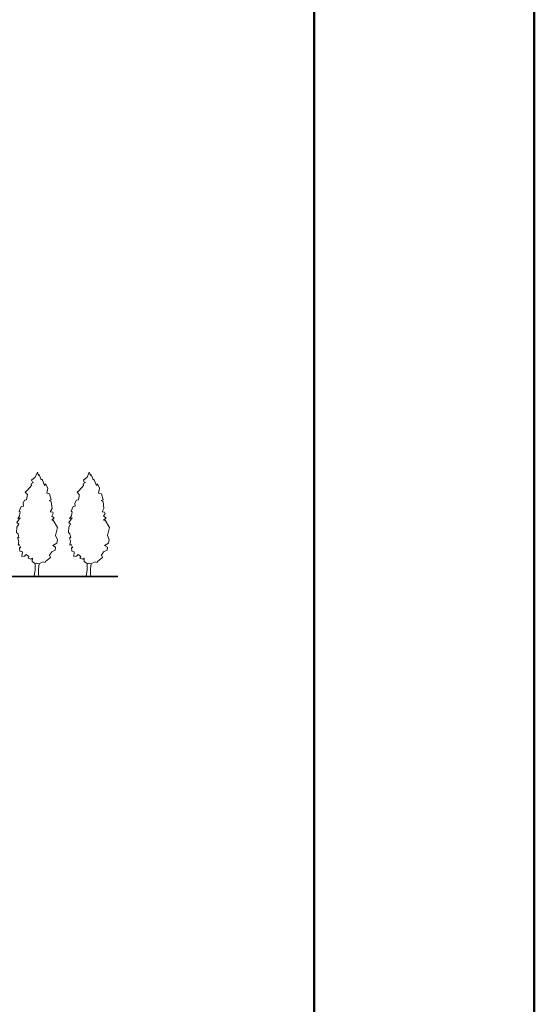
# Model space of a CAD drawing. Units: inches. Extents: x -1080 to 1950, y -1929 to 857.
# Tile 12 of 16: x 1630 to 1950, y -1001 to -389. Entities that reach past the tile are written whole.
import ezdxf

# ---------------------------------------------------------------- set-up
doc = ezdxf.new("R2010")
doc.units = ezdxf.units.IN
doc.header["$MEASUREMENT"] = 0
for name, color, linetype, lineweight in [('A-ANNO-TTLB', 7, 'Continuous', 50), ('A-ELEV', 7, 'Continuous', 35), ('L-PLNT', 82, 'Continuous', 13)]:
    doc.layers.add(name, color=color, linetype=linetype, lineweight=lineweight)

# ---------------------------------------------------------------- blocks, each defined once
blk = doc.blocks.new('*U5')
blk.add_lwpolyline([(-2.754, 191.699), (-6.78, 182.851), (-13.682, 176.953), (-11.956, 173.266), (-9.656, 172.529), (-14.257, 170.317), (-13.682, 167.368), (-21.733, 157.783), (-25.184, 154.834), (-21.158, 150.41), (-21.733, 147.461), (-22.884, 140.825), (-26.334, 140.087), (-29.21, 134.926), (-28.635, 129.028), (-32.661, 128.291), (-36.111, 120.18), (-34.386, 118.706), (-35.536, 111.333), (-38.987, 106.171), (-34.386, 107.646), (-40.712, 98.798), (-37.261, 95.849), (-40.712, 90.688), (-41.287, 80.366), (-38.412, 78.154), (-36.686, 70.781), (-39.562, 71.518), (-37.261, 64.145), (-38.412, 57.509), (-36.111, 58.247), (-33.236, 52.348), (-35.536, 53.086), (-34.961, 46.45), (-30.36, 44.975), (-31.51, 36.128), (-26.334, 36.865), (-23.459, 39.814), (-18.283, 36.128), (-20.008, 33.178), (-14.832, 31.704), (-11.956, 33.178), (-12.531, 27.28), (-6.205, 22.856), (-3.905, 24.331), (0.121, 22.856), (8.173, 26.543), (11.624, 25.068), (12.199, 27.28), (21.4, 34.653), (19.675, 39.077), (23.701, 44.975), (30.027, 47.924), (30.602, 53.823), (25.426, 56.772), (32.903, 61.196), (34.053, 67.094), (30.602, 75.205), (34.628, 89.951), (26.576, 103.222), (23.701, 103.222), (28.302, 107.646), (23.701, 110.595), (26.576, 115.756), (25.426, 117.968), (20.825, 118.706), (24.276, 124.604), (22.551, 137.876), (19.1, 139.35), (22.551, 140.825), (19.675, 151.884), (14.499, 153.359), (16.224, 162.207), (12.199, 170.317), (10.473, 167.368), (5.872, 179.165), (4.147, 177.69), (0.696, 187.275), (-0.454, 185.8)], close=True)
for points in [[(-6.813, 23.669), (-6.813, 11.669), (-8.627, 0)], [(0.387, 23.669), (-0.576, 13.271), (-0.576, 3.686), (0, 0)]]:
    blk.add_lwpolyline(points)

msp = doc.modelspace()

# ---------------------------------------------------------------- linework, layer by layer
at = {"layer": 'A-ANNO-TTLB'}
for points in [[(-1080.09, 856.52), (1950.41, 856.52), (1950.41, -1928.98), (-1080.09, -1928.98)], [(-957.59, 743.52), (1813.41, 743.52), (1813.41, -1770.48), (-957.59, -1770.48)]]:
    msp.add_lwpolyline(points, close=True, dxfattribs=at)
at = {"layer": 'A-ELEV'}
msp.add_line((1442.74, -734.72), (1691.4, -734.72), dxfattribs=at)

# ---------------------------------------------------------------- block references
at = {"layer": 'L-PLNT', "xscale": 0.3373382957572102, "yscale": 0.3373382957572102, "zscale": 0.3373382957572102}
for p in [(1642.24, -734.62), (1674.53, -734.62)]:
    msp.add_blockref('*U5', p, dxfattribs=at)

doc.saveas('drawing.dxf')
